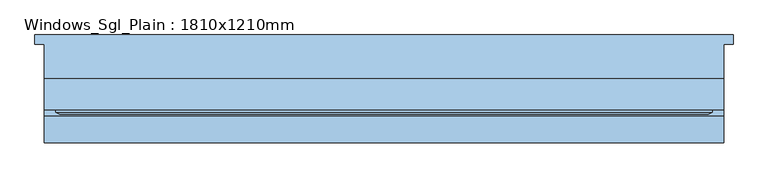
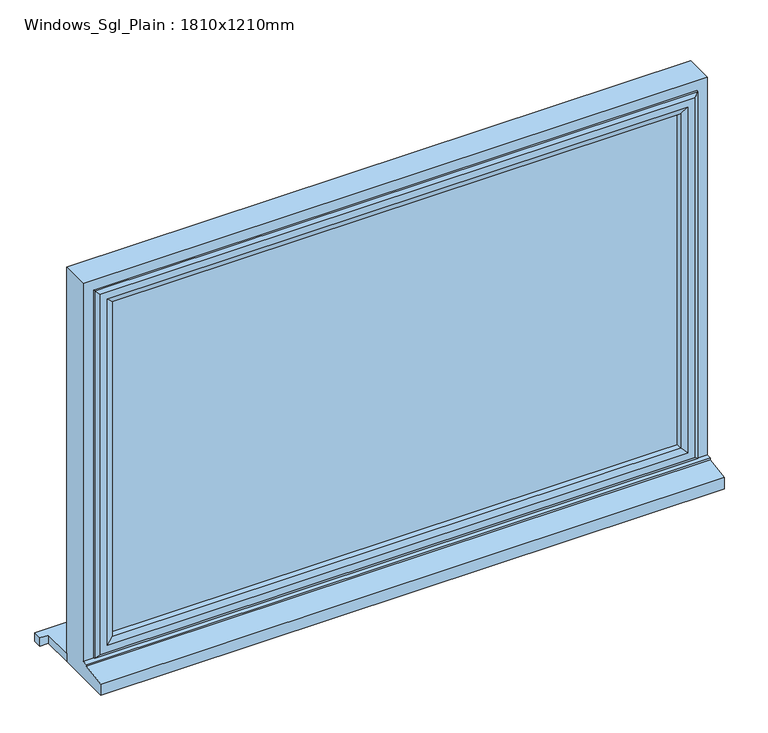
"""IFC4 building model written with IfcOpenShell, lengths in millimetres: window geometry, Windows_Sgl_Plain : 1810x1210mm."""

from ifc_helpers import new_model, si_unit, frame, origin, place, context, project, spatial, polyline, outline, extrude, faceted_brep, source, transform, mapped, element, save


def windows_sgl_plain_1810x1210mm_541be4ad(model_context):
    return source(origin(), model_context, "Body", "SolidModel", [
        extrude(outline(polyline([(-930.0, 129.0434322), (930.0, 129.0434322), (930.0, 104.0434322), (905.0, 104.0434322), (905.0, 12.0434322), (-905.0, 12.0434322), (-905.0, 104.0434322), (-930.0, 104.0434322), (-930.0, 129.0434322)])), frame((0.0, 0.0, 900.0), z_axis=(0.0, 0.0, 1.0), x_axis=(1.0, 0.0, 0.0)), (0.0, 0.0, 1.0), 25.0),
        faceted_brep([(-905.0, 12.0434322, 900.0), (-905.0, 12.0434322, 2110.0), (905.0, 12.0434322, 2110.0), (905.0, 12.0434322, 900.0), (-845.0, 12.0434322, 2050.0), (-845.0, 12.0434322, 975.0), (845.0, 12.0434322, 975.0), (845.0, 12.0434322, 2050.0), (-905.0, -158.4565678, 900.0), (-905.0, -158.4565678, 933.8088847), (-905.0, -85.9565678, 944.7449676), (-905.0, -85.9565678, 949.68767), (-905.0, -70.9565678, 951.0), (-905.0, -70.9565678, 2110.0), (905.0, -70.9565678, 951.0), (905.0, -70.9565678, 2110.0), (-865.0, -70.9565678, 2070.0), (865.0, -70.9565678, 2070.0), (865.0, -70.9565678, 963.0), (-865.0, -70.9565678, 963.0), (-865.0, -5.9565678, 963.0), (-865.0, -5.9565678, 2070.0), (865.0, -5.9565678, 963.0), (865.0, -5.9565678, 2070.0), (-845.0, -5.9565678, 2050.0), (845.0, -5.9565678, 2050.0), (845.0, -5.9565678, 975.0), (-845.0, -5.9565678, 975.0), (905.0, -85.9565678, 949.68767), (905.0, -85.9565678, 944.7449676), (905.0, -158.4565678, 933.8088847), (905.0, -158.4565678, 900.0)], [[[0, 1, 2, 3], [4, 5, 6, 7]], [[0, 8, 9, 10, 11, 12, 13, 1]], [[12, 14, 15, 13], [16, 17, 18, 19]], [[19, 20, 21, 16]], [[21, 20, 22, 23], [24, 25, 26, 27]], [[24, 27, 5, 4]], [[1, 13, 15, 2]], [[16, 21, 23, 17]], [[7, 25, 24, 4]], [[14, 28, 29, 30, 31, 3, 2, 15]], [[17, 23, 22, 18]], [[7, 6, 26, 25]], [[31, 8, 0, 3]], [[30, 9, 8, 31]], [[29, 10, 9, 30]], [[28, 11, 10, 29]], [[14, 12, 11, 28]], [[20, 19, 18, 22]], [[5, 27, 26, 6]]]),
        extrude(outline(polyline([(835.0, -34.9565678), (835.0, -58.9565678), (-835.0, -58.9565678), (-835.0, -34.9565678), (835.0, -34.9565678)])), frame((0.0, 0.0, 993.0), z_axis=(0.0, 0.0, 1.0), x_axis=(1.0, 0.0, 0.0)), (0.0, 0.0, 1.0), 1047.0),
        faceted_brep([(-875.0, -70.9565678, 2080.0), (-875.0, -70.9565678, 953.0), (-875.0, -76.7300705, 953.0), (-875.0, -76.7300705, 2080.0), (-865.0, -5.9565678, 2070.0), (-865.0, -5.9565678, 963.0), (-865.0, -70.9565678, 963.0), (-865.0, -70.9565678, 2070.0), (-825.0, -20.4494677, 2030.0), (-825.0, -20.4494677, 1003.0), (-835.1480377, -5.9565678, 992.8519623), (-835.1480377, -5.9565678, 2040.1480377), (-825.0, -34.9565678, 2030.0), (-825.0, -34.9565678, 1003.0), (-835.0, -58.9565678, 2040.0), (-835.0, -58.9565678, 993.0), (-835.0, -34.9565678, 993.0), (-835.0, -34.9565678, 2040.0), (-825.0, -76.7300705, 2030.0), (-825.0, -76.7300705, 1003.0), (-825.0, -58.9565678, 1003.0), (-825.0, -58.9565678, 2030.0), (-842.4457548, -82.5035732, 2047.4457548), (-842.4457548, -82.5035732, 985.5542452), (-864.2153903, -82.5035732, 963.7846097), (-864.2153903, -82.5035732, 2069.2153903), (875.0, -70.9565678, 953.0), (875.0, -76.7300705, 953.0), (865.0, -5.9565678, 963.0), (865.0, -70.9565678, 963.0), (825.0, -20.4494677, 1003.0), (835.1480377, -5.9565678, 992.8519623), (825.0, -34.9565678, 1003.0), (835.0, -58.9565678, 993.0), (835.0, -34.9565678, 993.0), (825.0, -76.7300705, 1003.0), (825.0, -58.9565678, 1003.0), (842.4457548, -82.5035732, 985.5542452), (864.2153903, -82.5035732, 963.7846097), (875.0, -70.9565678, 2080.0), (875.0, -76.7300705, 2080.0), (865.0, -5.9565678, 2070.0), (865.0, -70.9565678, 2070.0), (825.0, -20.4494677, 2030.0), (835.1480377, -5.9565678, 2040.1480377), (825.0, -34.9565678, 2030.0), (835.0, -58.9565678, 2040.0), (835.0, -34.9565678, 2040.0), (825.0, -76.7300705, 2030.0), (825.0, -58.9565678, 2030.0), (842.4457548, -82.5035732, 2047.4457548), (864.2153903, -82.5035732, 2069.2153903)], [[[0, 1, 2, 3]], [[4, 5, 6, 7]], [[8, 9, 10, 11]], [[12, 13, 9, 8]], [[14, 15, 16, 17]], [[18, 19, 20, 21]], [[22, 23, 19, 18]], [[3, 2, 24, 25]], [[1, 26, 27, 2]], [[5, 28, 29, 6]], [[9, 30, 31, 10]], [[13, 32, 30, 9]], [[15, 33, 34, 16]], [[19, 35, 36, 20]], [[23, 37, 35, 19]], [[2, 27, 38, 24]], [[26, 39, 40, 27]], [[28, 41, 42, 29]], [[30, 43, 44, 31]], [[32, 45, 43, 30]], [[33, 46, 47, 34]], [[35, 48, 49, 36]], [[37, 50, 48, 35]], [[27, 40, 51, 38]], [[39, 0, 3, 40]], [[1, 0, 39, 26], [7, 6, 29, 42]], [[41, 4, 7, 42]], [[5, 4, 41, 28], [11, 10, 31, 44]], [[43, 8, 11, 44]], [[45, 12, 8, 43]], [[17, 16, 34, 47], [13, 12, 45, 32]], [[46, 14, 17, 47]], [[15, 14, 46, 33], [21, 20, 36, 49]], [[48, 18, 21, 49]], [[50, 22, 18, 48]], [[25, 24, 38, 51], [23, 22, 50, 37]], [[40, 3, 25, 51]]]),
    ])


if __name__ == "__main__":
    model = new_model("IFC4")
    model_context = context("Model", 3, world=origin())
    ifc_project = project(units=[si_unit("LENGTHUNIT", "METRE", prefix="MILLI")], contexts=[model_context])
    site = spatial("IfcSite", under=ifc_project)
    building = spatial("IfcBuilding", under=site)
    placement = place(None, origin())
    windows_sgl_plain_1810x1210mm_shape = windows_sgl_plain_1810x1210mm_541be4ad(model_context)
    element("IfcWindow", 1, ObjectType="Windows_Sgl_Plain : 1810x1210mm", at=placement, inside=building, context=model_context, shape_type="MappedRepresentation", body=[
        mapped(windows_sgl_plain_1810x1210mm_shape, transform((0.0, 0.0, 0.0), x_axis=(1.0, 0.0, 0.0), y_axis=(0.0, 1.0, 0.0), z_axis=(0.0, 0.0, 1.0))),
    ])
    save(model, "model.ifc")

# Revit data of these elements
# Type "Windows_Sgl_Plain : 1810x1210mm"
#   Type Mark = "49"
#   Operation = "SinglePanel"
#   Construction Type Id = "SGL"
#   Manufacturer = "Revit"
#   Keynote = "L10"
#   Analytic Construction = "Large single-glazed windows"
#   Wrap Layers (Ext) from Ext = 102.5 mm
#   Wrap Layers (Int) from Ext = 177.5 mm
#   Window Board Projection = 25 mm
#   Window Board Extension = 25 mm
#   Visual Light Transmittance = 0.9
#   Solar Heat Gain Coefficient = 0.86
#   Rough Width = 1810 mm
#   Rough Height = 1210 mm
#   Height = 1210 mm
#   Width = 1810 mm
#   Heat Transfer Coefficient (U) = 5.5617 W/(m²·K)
#   Glazing Thickness = 24 mm
#   FrameOffset - External = 50 mm
#   Frame Depth = 65 mm
#   Default Head Height = 2110 mm
#   Cill Depth = 87.5 mm
#   Cavity Closer Width = 50 mm
#   Cavity Closer Offset from Ext = 102.5 mm
#   Cavity Closer Depth = 85 mm
#   Define Thermal Properties by = 1
#   Vis - Cavity Closers = yes
#   Define Thermal Properties by = 1
#   Material Trim = Window Frame
#   Material Glass = Glass
#   Material Frame = Window Frame
#   Wall Closure = (empty or 0)
# Element 1 (IfcWindow, "Windows_Sgl_Plain : 1810x1210mm")
#   Materials on its faces: "Window Frame", "Glass"
# Materials
#   "Window Frame": colour RGB 249 249 249, transparency 0, Keynote = "L10", Cost = 0
#   "Glass": class "Glass", colour RGB 0 128 192, transparency 0.9, Description = "Soda Lime Glass", Cost = 0
